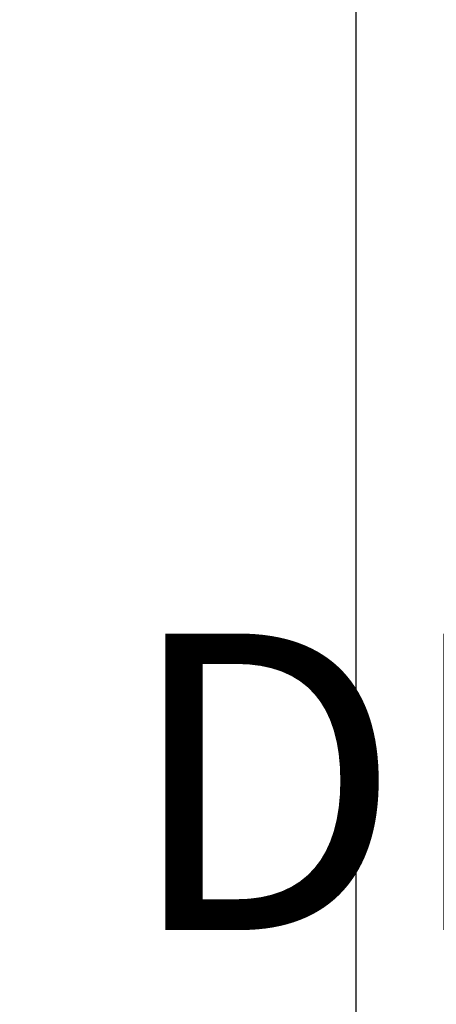
# Model space of a CAD drawing. Units: inches. Extents: x 305 to 776, y 38 to 479.
# Tile 6 of 14: x 350 to 378, y 265 to 332. Entities that reach past the tile are written whole.
import ezdxf

# ---------------------------------------------------------------- set-up
doc = ezdxf.new("R2010")
doc.units = ezdxf.units.IN
doc.header["$MEASUREMENT"] = 0
doc.layers.add('A-ANNO-DIMS', color=2, linetype='Continuous', lineweight=18)
doc.styles.get("Standard").update_dxf_attribs({"font": 'arial.ttf'})
doc.dimstyles.get("Standard").update_dxf_attribs({"dimtxt": 20, "dimasz": 0.18, "dimexe": 0.18, "dimexo": 0.0625, "dimgap": 0.09, "dimtad": 0, "dimtih": 1, "dimtoh": 1, "dimdec": 4, "dimzin": 0, "dimdsep": 46, "dimtxsty": 'Standard', "dimcen": 0.09, "dimadec": 0, "dimazin": 0, "dimtfac": 1, "dimtdec": 4, "dimtofl": 0, "dimtmove": 0, "dimatfit": 3, "dimfxl": 1, "dimtolj": 1, "dimtzin": 0, "dimarcsym": 0})

# ---------------------------------------------------------------- blocks, each defined once
blk = doc.blocks.new('*D33')
at = {"layer": 'A-ANNO-DIMS', "color": 0, "lineweight": -2, "transparency": 16777216}
for p, q in [((440.927, 307.949), (449.29, 307.949)), ((449.11, 307.769), (449.11, 290.896)), ((449.11, 253.161), (449.11, 270.034)), ((440.927, 252.981), (449.29, 252.981))]:
    blk.add_line(p, q, dxfattribs=at)
at = {"layer": 'A-ANNO-DIMS', "color": 0, "transparency": 16777216}
for points in [[(449.08, 307.769), (449.14, 307.769), (449.11, 307.949)], [(449.08, 253.161), (449.14, 253.161), (449.11, 252.981)]]:
    blk.add_solid(points, dxfattribs=at)
at = {"layer": 'Defpoints', "color": 0, "transparency": 16777216}
for p in [(440.864, 307.949), (449.11, 307.949), (440.864, 252.981)]:
    blk.add_point(p, dxfattribs=at)
at = {"layer": 'A-ANNO-DIMS', "color": 0, "transparency": 16777216, "insert": (449.11, 280.465), "char_height": 20, "attachment_point": 5}
blk.add_mtext('\\A1;DINING SET 55', dxfattribs=at)
blk = doc.blocks.new('*D46')
at = {"layer": 'A-ANNO-DIMS', "color": 0, "lineweight": -2, "transparency": 16777216}
for p, q in [((390.57, 429.382), (372.451, 429.382)), ((372.631, 429.202), (372.631, 259.69)), ((372.631, 69.562), (372.631, 239.074)), ((390.57, 69.382), (372.451, 69.382))]:
    blk.add_line(p, q, dxfattribs=at)
at = {"layer": 'A-ANNO-DIMS', "color": 0, "transparency": 16777216}
for points in [[(372.601, 429.202), (372.661, 429.202), (372.631, 429.382)], [(372.601, 69.562), (372.661, 69.562), (372.631, 69.382)]]:
    blk.add_solid(points, dxfattribs=at)
at = {"layer": 'Defpoints', "color": 0, "transparency": 16777216}
for p in [(372.631, 429.382), (390.633, 429.382), (390.633, 69.382)]:
    blk.add_point(p, dxfattribs=at)
at = {"layer": 'A-ANNO-DIMS', "color": 0, "transparency": 16777216, "insert": (372.631, 249.382), "char_height": 20, "attachment_point": 5}
blk.add_mtext('\\A1;360', dxfattribs=at)

msp = doc.modelspace()

# ---------------------------------------------------------------- dimensions: what is measured, and where the dimension line sits
at = {"layer": 'A-ANNO-DIMS'}
dim = msp.add_linear_dim(base=(372.6314, 429.382), p1=(390.6329, 69.382), p2=(390.6329, 429.382), angle=90, dimstyle='Standard', override={"dimdec": 0, "dimlfac": 1, "dimrnd": 0, "dimzin": 0, "dimdsep": 46, "dimlunit": 2}, dxfattribs=at)
dim.commit()
dim.dimension.update_dxf_attribs({"geometry": '*D46', "text_midpoint": (372.6314, 249.382)})
dim = msp.add_linear_dim(base=(449.1096, 307.9493), p1=(440.8644, 252.9815), p2=(440.8644, 307.9493), angle=90, text='DINING SET <>', dimstyle='Standard', override={"dimdec": 0, "dimlfac": 1, "dimrnd": 0, "dimzin": 0, "dimdsep": 46, "dimlunit": 2}, dxfattribs=at)
dim.commit()
dim.dimension.update_dxf_attribs({"geometry": '*D33', "text_midpoint": (449.1096, 280.4654)})

doc.saveas('drawing.dxf')
